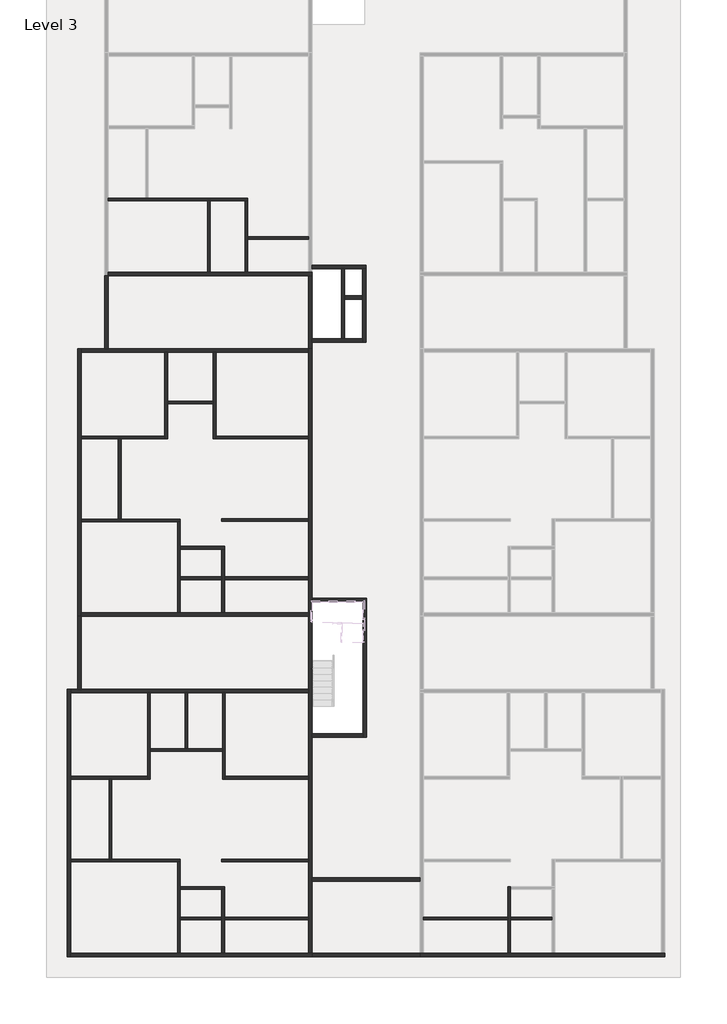
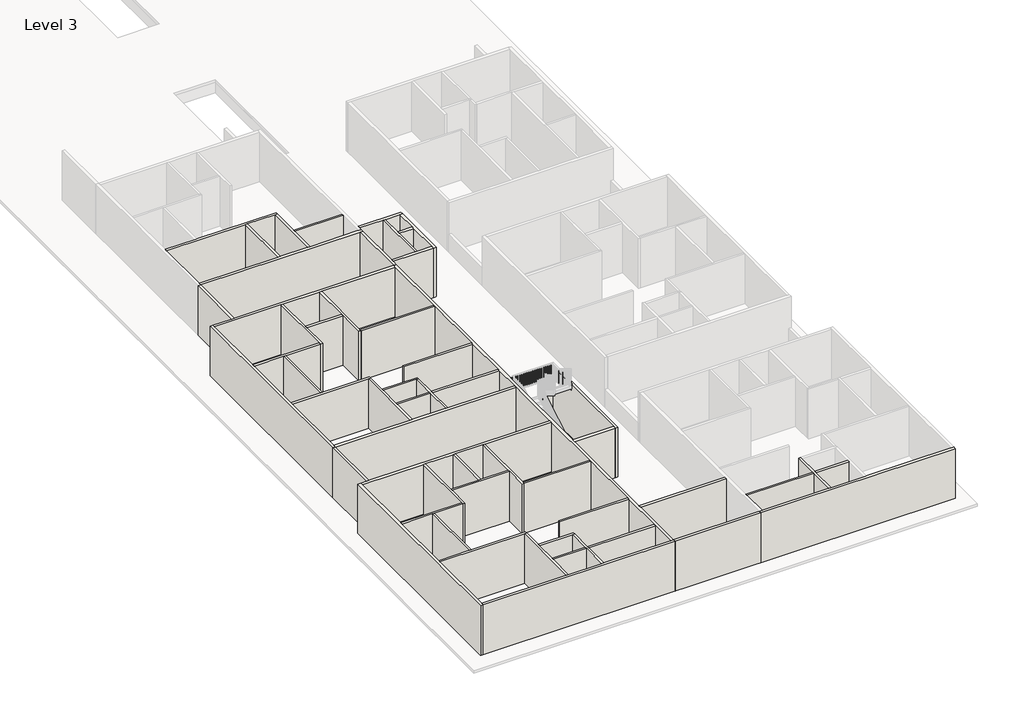
# One storey, part 1 of 8: 55 walls.
"""IFC4 building model written with IfcOpenShell, lengths in millimetres."""

from ifc_helpers import new_model, si_unit, frame, origin, place, context, project, spatial, polyline, outline, extrude, faceted_brep, element, save

model = new_model("IFC4")

# Units and contexts
model_context = context("Model", 3, world=origin())
ifc_project = project(units=[si_unit("LENGTHUNIT", "METRE", prefix="MILLI")], contexts=[model_context])

# Site, building, storey
site = spatial("IfcSite", under=ifc_project)
building = spatial("IfcBuilding", under=site)
storey = spatial("IfcBuildingStorey", under=building, Name="Level 3", Elevation=31330.6172466)

# Walls
placement = place(None, origin())
element("IfcWall", 1, ObjectType="4.5\"", at=placement, inside=storey, context=model_context, shape_type="Brep", body=[
    faceted_brep([(-12531.5544854, -1061.7344126, 31330.6172466), (-8188.1544854, -1061.7344126, 31330.6172466), (-8073.8544854, -1061.7344126, 31330.6172466), (-6549.8544854, -1061.7344126, 31330.6172466), (-6435.5544854, -1061.7344126, 31330.6172466), (-6435.5544854, -1061.7344126, 34378.6172466), (-6549.8544854, -1061.7344126, 34378.6172466), (-8073.8544854, -1061.7344126, 34378.6172466), (-8188.1544854, -1061.7344126, 34378.6172466), (-12531.5544854, -1061.7344126, 34378.6172466), (-12531.5544854, -947.4344126, 31330.6172466), (-12531.5544854, -947.4344126, 34378.6172466), (-10907.2415084, -947.4344126, 34378.6172466), (-10792.9415084, -947.4344126, 34378.6172466), (-6435.5544854, -947.4344126, 34378.6172466), (-6435.5544854, -947.4344126, 31330.6172466), (-10792.9415084, -947.4344126, 31330.6172466), (-10907.2415084, -947.4344126, 31330.6172466)], [[[0, 1, 2, 3, 4, 5, 6, 7, 8, 9]], [[10, 11, 12, 13, 14, 15, 16, 17]], [[4, 3, 2, 1, 0, 10, 17, 16, 15]], [[0, 9, 11, 10]], [[5, 4, 15, 14]], [[9, 8, 7, 6, 5, 14, 13, 12, 11]]]),
])
element("IfcWall", 2, ObjectType="4.5\"", at=placement, inside=storey, context=model_context, shape_type="Brep", body=[
    faceted_brep([(-6549.8544854, -1061.7344126, 31330.6172466), (-6549.8544854, -4185.9344126, 31330.6172466), (-6549.8544854, -4185.9344126, 34378.6172466), (-6549.8544854, -1061.7344126, 34378.6172466), (-6435.5544854, -1061.7344126, 31330.6172466), (-6435.5544854, -1061.7344126, 34378.6172466), (-6435.5544854, -2623.8344126, 34378.6172466), (-6435.5544854, -2738.1344126, 34378.6172466), (-6435.5544854, -4185.9344126, 34378.6172466), (-6435.5544854, -4185.9344126, 31330.6172466), (-6435.5544854, -2738.1344126, 31330.6172466), (-6435.5544854, -2623.8344126, 31330.6172466)], [[[0, 1, 2, 3]], [[4, 5, 6, 7, 8, 9, 10, 11]], [[1, 0, 4, 11, 10, 9]], [[0, 3, 5, 4]], [[2, 1, 9, 8]], [[3, 2, 8, 7, 6, 5]]]),
])
element("IfcWall", 3, ObjectType="4.5\"", at=placement, inside=storey, context=model_context, shape_type="SweptSolid", body=[
    extrude(outline(polyline([(-8188.1544854, -4185.9344126), (-8188.1544854, -1061.7344126), (-8073.8544854, -1061.7344126), (-8073.8544854, -4185.9344126), (-8188.1544854, -4185.9344126)])), frame((0.0, 0.0, 31330.6172466), z_axis=(0.0, 0.0, 1.0), x_axis=(1.0, 0.0, 0.0)), (0.0, 0.0, 1.0), 3048.0),
])
element("IfcWall", 4, ObjectType="4.5\"", at=placement, inside=storey, context=model_context, shape_type="SweptSolid", body=[
    extrude(outline(polyline([(-6435.5544854, -2623.8344126), (-3769.8415084, -2623.8344126), (-3769.8415084, -2738.1344126), (-6435.5544854, -2738.1344126), (-6435.5544854, -2623.8344126)])), frame((0.0, 0.0, 31330.6172466), z_axis=(0.0, 0.0, 1.0), x_axis=(1.0, 0.0, 0.0)), (0.0, 0.0, 1.0), 3048.0),
])
element("IfcWall", 5, ObjectType="4.5\"", at=placement, inside=storey, context=model_context, shape_type="Brep", body=[
    faceted_brep([(-10061.4044854, -7691.1344126, 31330.6172466), (-10061.4044854, -11348.7344126, 31330.6172466), (-10061.4044854, -11463.0344126, 31330.6172466), (-10061.4044854, -11463.0344126, 34378.6172466), (-10061.4044854, -11348.7344126, 34378.6172466), (-10061.4044854, -7691.1344126, 34378.6172466), (-9947.1044854, -7691.1344126, 31330.6172466), (-9947.1044854, -7691.1344126, 34378.6172466), (-9947.1044854, -9824.7344126, 34378.6172466), (-9947.1044854, -9939.0344126, 34378.6172466), (-9947.1044854, -11463.0344126, 34378.6172466), (-9947.1044854, -11463.0344126, 31330.6172466), (-9947.1044854, -9939.0344126, 31330.6172466), (-9947.1044854, -9824.7344126, 31330.6172466)], [[[0, 1, 2, 3, 4, 5]], [[6, 7, 8, 9, 10, 11, 12, 13]], [[2, 1, 0, 6, 13, 12, 11]], [[0, 5, 7, 6]], [[3, 2, 11, 10]], [[5, 4, 3, 10, 9, 8, 7]]]),
])
element("IfcWall", 6, ObjectType="4.5\"", at=placement, inside=storey, context=model_context, shape_type="Brep", body=[
    faceted_brep([(-10061.4044854, -11348.7344126, 31330.6172466), (-13719.0044854, -11348.7344126, 31330.6172466), (-13719.0044854, -11348.7344126, 34378.6172466), (-10061.4044854, -11348.7344126, 34378.6172466), (-10061.4044854, -11463.0344126, 31330.6172466), (-10061.4044854, -11463.0344126, 34378.6172466), (-11980.3915084, -11463.0344126, 34378.6172466), (-12094.6915084, -11463.0344126, 34378.6172466), (-13719.0044854, -11463.0344126, 34378.6172466), (-13719.0044854, -11463.0344126, 31330.6172466), (-12094.6915084, -11463.0344126, 31330.6172466), (-11980.3915084, -11463.0344126, 31330.6172466)], [[[0, 1, 2, 3]], [[4, 5, 6, 7, 8, 9, 10, 11]], [[1, 0, 4, 11, 10, 9]], [[0, 3, 5, 4]], [[2, 1, 9, 8]], [[3, 2, 8, 7, 6, 5]]]),
])
element("IfcWall", 7, ObjectType="4.5\"", at=placement, inside=storey, context=model_context, shape_type="SweptSolid", body=[
    extrude(outline(polyline([(-12094.6915084, -14968.2344126), (-12094.6915084, -11463.0344126), (-11980.3915084, -11463.0344126), (-11980.3915084, -14968.2344126), (-12094.6915084, -14968.2344126)])), frame((0.0, 0.0, 31330.6172466), z_axis=(0.0, 0.0, 1.0), x_axis=(1.0, 0.0, 0.0)), (0.0, 0.0, 1.0), 3048.0),
])
element("IfcWall", 8, ObjectType="4.5\"", at=placement, inside=storey, context=model_context, shape_type="Brep", body=[
    faceted_brep([(-13719.0044854, -15095.2344126, 31330.6172466), (-9510.2415084, -15095.2344126, 31330.6172466), (-9395.9415084, -15095.2344126, 31330.6172466), (-9395.9415084, -15095.2344126, 34378.6172466), (-9510.2415084, -15095.2344126, 34378.6172466), (-13719.0044854, -15095.2344126, 34378.6172466), (-13719.0044854, -14980.9344126, 31330.6172466), (-13719.0044854, -14980.9344126, 34378.6172466), (-9395.9415084, -14980.9344126, 34378.6172466), (-9395.9415084, -14980.9344126, 31330.6172466)], [[[0, 1, 2, 3, 4, 5]], [[6, 7, 8, 9]], [[2, 1, 0, 6, 9]], [[0, 5, 7, 6]], [[3, 2, 9, 8]], [[5, 4, 3, 8, 7]]]),
])
element("IfcWall", 9, ObjectType="4.5\"", at=placement, inside=storey, context=model_context, shape_type="Brep", body=[
    faceted_brep([(-9510.2415084, -15095.2344126, 31330.6172466), (-9510.2415084, -19070.3344126, 31330.6172466), (-9510.2415084, -19070.3344126, 34378.6172466), (-9510.2415084, -15095.2344126, 34378.6172466), (-9395.9415084, -15095.2344126, 31330.6172466), (-9395.9415084, -15095.2344126, 34378.6172466), (-9395.9415084, -16174.7344126, 34378.6172466), (-9395.9415084, -16289.0344126, 34378.6172466), (-9395.9415084, -17508.2344126, 34378.6172466), (-9395.9415084, -17622.5344126, 34378.6172466), (-9395.9415084, -19070.3344126, 34378.6172466), (-9395.9415084, -19070.3344126, 31330.6172466), (-9395.9415084, -17622.5344126, 31330.6172466), (-9395.9415084, -17508.2344126, 31330.6172466), (-9395.9415084, -16289.0344126, 31330.6172466), (-9395.9415084, -16174.7344126, 31330.6172466)], [[[0, 1, 2, 3]], [[4, 5, 6, 7, 8, 9, 10, 11, 12, 13, 14, 15]], [[1, 0, 4, 15, 14, 13, 12, 11]], [[0, 3, 5, 4]], [[2, 1, 11, 10]], [[3, 2, 10, 9, 8, 7, 6, 5]]]),
])
element("IfcWall", 10, ObjectType="4.5\"", at=placement, inside=storey, context=model_context, shape_type="Brep", body=[
    faceted_brep([(-9395.9415084, -16289.0344126, 31330.6172466), (-7567.1415084, -16289.0344126, 31330.6172466), (-7452.8415084, -16289.0344126, 31330.6172466), (-7452.8415084, -16289.0344126, 34378.6172466), (-7567.1415084, -16289.0344126, 34378.6172466), (-9395.9415084, -16289.0344126, 34378.6172466), (-9395.9415084, -16174.7344126, 31330.6172466), (-9395.9415084, -16174.7344126, 34378.6172466), (-7452.8415084, -16174.7344126, 34378.6172466), (-7452.8415084, -16174.7344126, 31330.6172466)], [[[0, 1, 2, 3, 4, 5]], [[6, 7, 8, 9]], [[2, 1, 0, 6, 9]], [[0, 5, 7, 6]], [[3, 2, 9, 8]], [[5, 4, 3, 8, 7]]]),
])
element("IfcWall", 11, ObjectType="4.5\"", at=placement, inside=storey, context=model_context, shape_type="Brep", body=[
    faceted_brep([(-7567.1415084, -16289.0344126, 31330.6172466), (-7567.1415084, -17508.2344126, 31330.6172466), (-7567.1415084, -17622.5344126, 31330.6172466), (-7567.1415084, -19070.3344126, 31330.6172466), (-7567.1415084, -19070.3344126, 34378.6172466), (-7567.1415084, -17622.5344126, 34378.6172466), (-7567.1415084, -17508.2344126, 34378.6172466), (-7567.1415084, -16289.0344126, 34378.6172466), (-7452.8415084, -16289.0344126, 31330.6172466), (-7452.8415084, -16289.0344126, 34378.6172466), (-7452.8415084, -17508.2344126, 34378.6172466), (-7452.8415084, -17622.5344126, 34378.6172466), (-7452.8415084, -19070.3344126, 34378.6172466), (-7452.8415084, -19070.3344126, 31330.6172466), (-7452.8415084, -17622.5344126, 31330.6172466), (-7452.8415084, -17508.2344126, 31330.6172466)], [[[0, 1, 2, 3, 4, 5, 6, 7]], [[8, 9, 10, 11, 12, 13, 14, 15]], [[3, 2, 1, 0, 8, 15, 14, 13]], [[0, 7, 9, 8]], [[4, 3, 13, 12]], [[7, 6, 5, 4, 12, 11, 10, 9]]]),
])
element("IfcWall", 12, ObjectType="4.5\"", at=placement, inside=storey, context=model_context, shape_type="SweptSolid", body=[
    extrude(outline(polyline([(-7567.1415084, -17622.5344126), (-9395.9415084, -17622.5344126), (-9395.9415084, -17508.2344126), (-7567.1415084, -17508.2344126), (-7567.1415084, -17622.5344126)])), frame((0.0, 0.0, 31330.6172466), z_axis=(0.0, 0.0, 1.0), x_axis=(1.0, 0.0, 0.0)), (0.0, 0.0, 1.0), 3048.0),
])
element("IfcWall", 13, ObjectType="4.5\"", at=placement, inside=storey, context=model_context, shape_type="SweptSolid", body=[
    extrude(outline(polyline([(-3769.8415084, -17622.5344126), (-7452.8415084, -17622.5344126), (-7452.8415084, -17508.2344126), (-3769.8415084, -17508.2344126), (-3769.8415084, -17622.5344126)])), frame((0.0, 0.0, 31330.6172466), z_axis=(0.0, 0.0, 1.0), x_axis=(1.0, 0.0, 0.0)), (0.0, 0.0, 1.0), 3048.0),
])
element("IfcWall", 14, ObjectType="4.5\"", at=placement, inside=storey, context=model_context, shape_type="SweptSolid", body=[
    extrude(outline(polyline([(-7567.1415084, -14968.2344126), (-3769.8415084, -14968.2344126), (-3769.8415084, -15082.5344126), (-7567.1415084, -15082.5344126), (-7567.1415084, -14968.2344126)])), frame((0.0, 0.0, 31330.6172466), z_axis=(0.0, 0.0, 1.0), x_axis=(1.0, 0.0, 0.0)), (0.0, 0.0, 1.0), 3048.0),
])
element("IfcWall", 15, ObjectType="4.5\"", at=placement, inside=storey, context=model_context, shape_type="SweptSolid", body=[
    extrude(outline(polyline([(-7940.5044854, -9939.0344126), (-9947.1044854, -9939.0344126), (-9947.1044854, -9824.7344126), (-7940.5044854, -9824.7344126), (-7940.5044854, -9939.0344126)])), frame((0.0, 0.0, 31330.6172466), z_axis=(0.0, 0.0, 1.0), x_axis=(1.0, 0.0, 0.0)), (0.0, 0.0, 1.0), 3048.0),
])
element("IfcWall", 16, ObjectType="4.5\"", at=placement, inside=storey, context=model_context, shape_type="Brep", body=[
    faceted_brep([(-7940.5044854, -7691.1344126, 31330.6172466), (-7940.5044854, -9824.7344126, 31330.6172466), (-7940.5044854, -9939.0344126, 31330.6172466), (-7940.5044854, -11463.0344126, 31330.6172466), (-7940.5044854, -11463.0344126, 34378.6172466), (-7940.5044854, -9939.0344126, 34378.6172466), (-7940.5044854, -9824.7344126, 34378.6172466), (-7940.5044854, -7691.1344126, 34378.6172466), (-7826.2044854, -7691.1344126, 31330.6172466), (-7826.2044854, -7691.1344126, 34378.6172466), (-7826.2044854, -11348.7344126, 34378.6172466), (-7826.2044854, -11463.0344126, 34378.6172466), (-7826.2044854, -11463.0344126, 31330.6172466), (-7826.2044854, -11348.7344126, 31330.6172466)], [[[0, 1, 2, 3, 4, 5, 6, 7]], [[8, 9, 10, 11, 12, 13]], [[3, 2, 1, 0, 8, 13, 12]], [[0, 7, 9, 8]], [[4, 3, 12, 11]], [[7, 6, 5, 4, 11, 10, 9]]]),
])
element("IfcWall", 17, ObjectType="4.5\"", at=placement, inside=storey, context=model_context, shape_type="SweptSolid", body=[
    extrude(outline(polyline([(-3769.8415084, -11463.0344126), (-7826.2044854, -11463.0344126), (-7826.2044854, -11348.7344126), (-3769.8415084, -11348.7344126), (-3769.8415084, -11463.0344126)])), frame((0.0, 0.0, 31330.6172466), z_axis=(0.0, 0.0, 1.0), x_axis=(1.0, 0.0, 0.0)), (0.0, 0.0, 1.0), 3048.0),
])
element("IfcWall", 18, ObjectType="4.5\"", at=placement, inside=storey, context=model_context, shape_type="Brep", body=[
    faceted_brep([(-10818.3415084, -22575.5344126, 31330.6172466), (-10818.3415084, -26233.1344126, 31330.6172466), (-10818.3415084, -26347.4344126, 31330.6172466), (-10818.3415084, -26347.4344126, 34378.6172466), (-10818.3415084, -26233.1344126, 34378.6172466), (-10818.3415084, -22575.5344126, 34378.6172466), (-10704.0415084, -22575.5344126, 31330.6172466), (-10704.0415084, -22575.5344126, 34378.6172466), (-10704.0415084, -25013.9344126, 34378.6172466), (-10704.0415084, -25128.2344126, 34378.6172466), (-10704.0415084, -26347.4344126, 34378.6172466), (-10704.0415084, -26347.4344126, 31330.6172466), (-10704.0415084, -25128.2344126, 31330.6172466), (-10704.0415084, -25013.9344126, 31330.6172466)], [[[0, 1, 2, 3, 4, 5]], [[6, 7, 8, 9, 10, 11, 12, 13]], [[2, 1, 0, 6, 13, 12, 11]], [[0, 5, 7, 6]], [[3, 2, 11, 10]], [[5, 4, 3, 10, 9, 8, 7]]]),
])
element("IfcWall", 19, ObjectType="4.5\"", at=placement, inside=storey, context=model_context, shape_type="Brep", body=[
    faceted_brep([(-10818.3415084, -26233.1344126, 31330.6172466), (-14171.1415084, -26233.1344126, 31330.6172466), (-14171.1415084, -26233.1344126, 34378.6172466), (-10818.3415084, -26233.1344126, 34378.6172466), (-10818.3415084, -26347.4344126, 31330.6172466), (-10818.3415084, -26347.4344126, 34378.6172466), (-12380.4415084, -26347.4344126, 34378.6172466), (-12494.7415084, -26347.4344126, 34378.6172466), (-14171.1415084, -26347.4344126, 34378.6172466), (-14171.1415084, -26347.4344126, 31330.6172466), (-12494.7415084, -26347.4344126, 31330.6172466), (-12380.4415084, -26347.4344126, 31330.6172466)], [[[0, 1, 2, 3]], [[4, 5, 6, 7, 8, 9, 10, 11]], [[1, 0, 4, 11, 10, 9]], [[0, 3, 5, 4]], [[2, 1, 9, 8]], [[3, 2, 8, 7, 6, 5]]]),
])
element("IfcWall", 20, ObjectType="4.5\"", at=placement, inside=storey, context=model_context, shape_type="SweptSolid", body=[
    extrude(outline(polyline([(-9180.0415084, -25013.9344126), (-9180.0415084, -22575.5344126), (-9065.7415084, -22575.5344126), (-9065.7415084, -25013.9344126), (-9180.0415084, -25013.9344126)])), frame((0.0, 0.0, 31330.6172466), z_axis=(0.0, 0.0, 1.0), x_axis=(1.0, 0.0, 0.0)), (0.0, 0.0, 1.0), 3048.0),
])
element("IfcWall", 21, ObjectType="4.5\"", at=placement, inside=storey, context=model_context, shape_type="Brep", body=[
    faceted_brep([(-10704.0415084, -25128.2344126, 31330.6172466), (-7541.7415084, -25128.2344126, 31330.6172466), (-7541.7415084, -25128.2344126, 34378.6172466), (-10704.0415084, -25128.2344126, 34378.6172466), (-10704.0415084, -25013.9344126, 31330.6172466), (-10704.0415084, -25013.9344126, 34378.6172466), (-9180.0415084, -25013.9344126, 34378.6172466), (-9065.7415084, -25013.9344126, 34378.6172466), (-7541.7415084, -25013.9344126, 34378.6172466), (-7541.7415084, -25013.9344126, 31330.6172466), (-9065.7415084, -25013.9344126, 31330.6172466), (-9180.0415084, -25013.9344126, 31330.6172466)], [[[0, 1, 2, 3]], [[4, 5, 6, 7, 8, 9, 10, 11]], [[1, 0, 4, 11, 10, 9]], [[0, 3, 5, 4]], [[2, 1, 9, 8]], [[3, 2, 8, 7, 6, 5]]]),
])
element("IfcWall", 22, ObjectType="4.5\"", at=placement, inside=storey, context=model_context, shape_type="Brep", body=[
    faceted_brep([(-7541.7415084, -22575.5344126, 31330.6172466), (-7541.7415084, -25013.9344126, 31330.6172466), (-7541.7415084, -25128.2344126, 31330.6172466), (-7541.7415084, -26347.4344126, 31330.6172466), (-7541.7415084, -26347.4344126, 34378.6172466), (-7541.7415084, -25128.2344126, 34378.6172466), (-7541.7415084, -25013.9344126, 34378.6172466), (-7541.7415084, -22575.5344126, 34378.6172466), (-7427.4415084, -22575.5344126, 31330.6172466), (-7427.4415084, -22575.5344126, 34378.6172466), (-7427.4415084, -26233.1344126, 34378.6172466), (-7427.4415084, -26347.4344126, 34378.6172466), (-7427.4415084, -26347.4344126, 31330.6172466), (-7427.4415084, -26233.1344126, 31330.6172466)], [[[0, 1, 2, 3, 4, 5, 6, 7]], [[8, 9, 10, 11, 12, 13]], [[3, 2, 1, 0, 8, 13, 12]], [[0, 7, 9, 8]], [[4, 3, 12, 11]], [[7, 6, 5, 4, 11, 10, 9]]]),
])
element("IfcWall", 23, ObjectType="4.5\"", at=placement, inside=storey, context=model_context, shape_type="SweptSolid", body=[
    extrude(outline(polyline([(-3769.8415084, -26347.4344126), (-7427.4415084, -26347.4344126), (-7427.4415084, -26233.1344126), (-3769.8415084, -26233.1344126), (-3769.8415084, -26347.4344126)])), frame((0.0, 0.0, 31330.6172466), z_axis=(0.0, 0.0, 1.0), x_axis=(1.0, 0.0, 0.0)), (0.0, 0.0, 1.0), 3048.0),
])
element("IfcWall", 24, ObjectType="4.5\"", at=placement, inside=storey, context=model_context, shape_type="SweptSolid", body=[
    extrude(outline(polyline([(-12494.7415084, -29852.6344126), (-12494.7415084, -26347.4344126), (-12380.4415084, -26347.4344126), (-12380.4415084, -29852.6344126), (-12494.7415084, -29852.6344126)])), frame((0.0, 0.0, 31330.6172466), z_axis=(0.0, 0.0, 1.0), x_axis=(1.0, 0.0, 0.0)), (0.0, 0.0, 1.0), 3048.0),
])
element("IfcWall", 25, ObjectType="4.5\"", at=placement, inside=storey, context=model_context, shape_type="Brep", body=[
    faceted_brep([(-14171.1415084, -29966.9344126, 31330.6172466), (-9510.2415084, -29966.9344126, 31330.6172466), (-9395.9415084, -29966.9344126, 31330.6172466), (-9395.9415084, -29966.9344126, 34378.6172466), (-9510.2415084, -29966.9344126, 34378.6172466), (-14171.1415084, -29966.9344126, 34378.6172466), (-14171.1415084, -29852.6344126, 31330.6172466), (-14171.1415084, -29852.6344126, 34378.6172466), (-12494.7415084, -29852.6344126, 34378.6172466), (-12380.4415084, -29852.6344126, 34378.6172466), (-9395.9415084, -29852.6344126, 34378.6172466), (-9395.9415084, -29852.6344126, 31330.6172466), (-12380.4415084, -29852.6344126, 31330.6172466), (-12494.7415084, -29852.6344126, 31330.6172466)], [[[0, 1, 2, 3, 4, 5]], [[6, 7, 8, 9, 10, 11, 12, 13]], [[2, 1, 0, 6, 13, 12, 11]], [[0, 5, 7, 6]], [[3, 2, 11, 10]], [[5, 4, 3, 10, 9, 8, 7]]]),
])
element("IfcWall", 26, ObjectType="4.5\"", at=placement, inside=storey, context=model_context, shape_type="Brep", body=[
    faceted_brep([(-9510.2415084, -29966.9344126, 31330.6172466), (-9510.2415084, -33954.7344126, 31330.6172466), (-9510.2415084, -33954.7344126, 34378.6172466), (-9510.2415084, -29966.9344126, 34378.6172466), (-9395.9415084, -29966.9344126, 31330.6172466), (-9395.9415084, -29966.9344126, 34378.6172466), (-9395.9415084, -31059.1344126, 34378.6172466), (-9395.9415084, -31173.4344126, 34378.6172466), (-9395.9415084, -32392.6344126, 34378.6172466), (-9395.9415084, -32506.9344126, 34378.6172466), (-9395.9415084, -33954.7344126, 34378.6172466), (-9395.9415084, -33954.7344126, 31330.6172466), (-9395.9415084, -32506.9344126, 31330.6172466), (-9395.9415084, -32392.6344126, 31330.6172466), (-9395.9415084, -31173.4344126, 31330.6172466), (-9395.9415084, -31059.1344126, 31330.6172466)], [[[0, 1, 2, 3]], [[4, 5, 6, 7, 8, 9, 10, 11, 12, 13, 14, 15]], [[1, 0, 4, 15, 14, 13, 12, 11]], [[0, 3, 5, 4]], [[2, 1, 11, 10]], [[3, 2, 10, 9, 8, 7, 6, 5]]]),
])
element("IfcWall", 27, ObjectType="4.5\"", at=placement, inside=storey, context=model_context, shape_type="Brep", body=[
    faceted_brep([(-9395.9415084, -31173.4344126, 31330.6172466), (-7567.1415084, -31173.4344126, 31330.6172466), (-7452.8415084, -31173.4344126, 31330.6172466), (-7452.8415084, -31173.4344126, 34378.6172466), (-7567.1415084, -31173.4344126, 34378.6172466), (-9395.9415084, -31173.4344126, 34378.6172466), (-9395.9415084, -31059.1344126, 31330.6172466), (-9395.9415084, -31059.1344126, 34378.6172466), (-7452.8415084, -31059.1344126, 34378.6172466), (-7452.8415084, -31059.1344126, 31330.6172466)], [[[0, 1, 2, 3, 4, 5]], [[6, 7, 8, 9]], [[2, 1, 0, 6, 9]], [[0, 5, 7, 6]], [[3, 2, 9, 8]], [[5, 4, 3, 8, 7]]]),
])
element("IfcWall", 28, ObjectType="4.5\"", at=placement, inside=storey, context=model_context, shape_type="Brep", body=[
    faceted_brep([(-7567.1415084, -31173.4344126, 31330.6172466), (-7567.1415084, -32392.6344126, 31330.6172466), (-7567.1415084, -32506.9344126, 31330.6172466), (-7567.1415084, -33954.7344126, 31330.6172466), (-7567.1415084, -33954.7344126, 34378.6172466), (-7567.1415084, -32506.9344126, 34378.6172466), (-7567.1415084, -32392.6344126, 34378.6172466), (-7567.1415084, -31173.4344126, 34378.6172466), (-7452.8415084, -31173.4344126, 31330.6172466), (-7452.8415084, -31173.4344126, 34378.6172466), (-7452.8415084, -32392.6344126, 34378.6172466), (-7452.8415084, -32506.9344126, 34378.6172466), (-7452.8415084, -33954.7344126, 34378.6172466), (-7452.8415084, -33954.7344126, 31330.6172466), (-7452.8415084, -32506.9344126, 31330.6172466), (-7452.8415084, -32392.6344126, 31330.6172466)], [[[0, 1, 2, 3, 4, 5, 6, 7]], [[8, 9, 10, 11, 12, 13, 14, 15]], [[3, 2, 1, 0, 8, 15, 14, 13]], [[0, 7, 9, 8]], [[4, 3, 13, 12]], [[7, 6, 5, 4, 12, 11, 10, 9]]]),
])
element("IfcWall", 29, ObjectType="4.5\"", at=placement, inside=storey, context=model_context, shape_type="SweptSolid", body=[
    extrude(outline(polyline([(-3769.8415084, -32392.6344126), (-3769.8415084, -32506.9344126), (-7452.8415084, -32506.9344126), (-7452.8415084, -32392.6344126), (-3769.8415084, -32392.6344126)])), frame((0.0, 0.0, 31330.6172466), z_axis=(0.0, 0.0, 1.0), x_axis=(1.0, 0.0, 0.0)), (0.0, 0.0, 1.0), 3048.0),
    extrude(outline(polyline([(-9395.9415084, -32506.9344126), (-9395.9415084, -32392.6344126), (-7567.1415084, -32392.6344126), (-7567.1415084, -32506.9344126), (-9395.9415084, -32506.9344126)])), frame((0.0, 0.0, 31330.6172466), z_axis=(0.0, 0.0, 1.0), x_axis=(1.0, 0.0, 0.0)), (0.0, 0.0, 1.0), 3048.0),
])
element("IfcWall", 30, ObjectType="4.5\"", at=placement, inside=storey, context=model_context, shape_type="SweptSolid", body=[
    extrude(outline(polyline([(-7567.1415084, -29852.6344126), (-3769.8415084, -29852.6344126), (-3769.8415084, -29966.9344126), (-7567.1415084, -29966.9344126), (-7567.1415084, -29852.6344126)])), frame((0.0, 0.0, 31330.6172466), z_axis=(0.0, 0.0, 1.0), x_axis=(1.0, 0.0, 0.0)), (0.0, 0.0, 1.0), 3048.0),
])
element("IfcWall", 31, ObjectType="4.5\"", at=placement, inside=storey, context=model_context, shape_type="SweptSolid", body=[
    extrude(outline(polyline([(4942.3584916, -32506.9344126), (1259.3584916, -32506.9344126), (1259.3584916, -32392.6344126), (4942.3584916, -32392.6344126), (4942.3584916, -32506.9344126)])), frame((0.0, 0.0, 31330.6172466), z_axis=(0.0, 0.0, 1.0), x_axis=(1.0, 0.0, 0.0)), (0.0, 0.0, 1.0), 3048.0),
])
element("IfcWall", 32, ObjectType="4.5\"", at=placement, inside=storey, context=model_context, shape_type="Brep", body=[
    faceted_brep([(4942.3584916, -31059.1344126, 31330.6172466), (4942.3584916, -32392.6344126, 31330.6172466), (4942.3584916, -32506.9344126, 31330.6172466), (4942.3584916, -33954.7344126, 31330.6172466), (4942.3584916, -33954.7344126, 34378.6172466), (4942.3584916, -32506.9344126, 34378.6172466), (4942.3584916, -32392.6344126, 34378.6172466), (4942.3584916, -31059.1344126, 34378.6172466), (5056.6584916, -31059.1344126, 31330.6172466), (5056.6584916, -31059.1344126, 34378.6172466), (5056.6584916, -31173.4344126, 34378.6172466), (5056.6584916, -32392.6344126, 34378.6172466), (5056.6584916, -32506.9344126, 34378.6172466), (5056.6584916, -33954.7344126, 34378.6172466), (5056.6584916, -33954.7344126, 31330.6172466), (5056.6584916, -32506.9344126, 31330.6172466), (5056.6584916, -32392.6344126, 31330.6172466), (5056.6584916, -31173.4344126, 31330.6172466)], [[[0, 1, 2, 3, 4, 5, 6, 7]], [[8, 9, 10, 11, 12, 13, 14, 15, 16, 17]], [[3, 2, 1, 0, 8, 17, 16, 15, 14]], [[4, 3, 14, 13]], [[0, 7, 9, 8]], [[7, 6, 5, 4, 13, 12, 11, 10, 9]]]),
])
element("IfcWall", 33, ObjectType="4.5\"", at=placement, inside=storey, context=model_context, shape_type="SweptSolid", body=[
    extrude(outline(polyline([(6885.4584916, -32506.9344126), (5056.6584916, -32506.9344126), (5056.6584916, -32392.6344126), (6885.4584916, -32392.6344126), (6885.4584916, -32506.9344126)])), frame((0.0, 0.0, 31330.6172466), z_axis=(0.0, 0.0, 1.0), x_axis=(1.0, 0.0, 0.0)), (0.0, 0.0, 1.0), 3048.0),
])
element("IfcWall", 34, ObjectType="4.5\"", at=placement, inside=storey, context=model_context, shape_type="Brep", body=[
    faceted_brep([(-2207.6738684, -7082.6751812, 31330.6172466), (-2207.6738684, -5366.3479894, 31330.6172466), (-2207.6738684, -5213.9479894, 31330.6172466), (-2207.6738684, -4034.6751812, 31330.6172466), (-2207.6738684, -4034.6751812, 34378.6172466), (-2207.6738684, -5213.9479894, 34378.6172466), (-2207.6738684, -5366.3479894, 34378.6172466), (-2207.6738684, -7082.6751812, 34378.6172466), (-2321.9738684, -7082.6751812, 31330.6172466), (-2321.9738684, -7082.6751812, 34378.6172466), (-2321.9738684, -4034.6751812, 34378.6172466), (-2321.9738684, -4034.6751812, 31330.6172466)], [[[0, 1, 2, 3, 4, 5, 6, 7]], [[8, 9, 10, 11]], [[3, 2, 1, 0, 8, 11]], [[7, 6, 5, 4, 10, 9]], [[4, 3, 11, 10]], [[0, 7, 9, 8]]]),
])
element("IfcWall", 35, ObjectType="6\"", at=placement, inside=storey, context=model_context, shape_type="Brep", body=[
    faceted_brep([(-12531.5544854, -4338.3344126, 31330.6172466), (-3769.8415084, -4338.3344126, 31330.6172466), (-3617.4415084, -4338.3344126, 31330.6172466), (-3617.4415084, -4338.3344126, 34378.6172466), (-3769.8415084, -4338.3344126, 34378.6172466), (-12531.5544854, -4338.3344126, 34378.6172466), (-12531.5544854, -4185.9344126, 31330.6172466), (-12531.5544854, -4185.9344126, 34378.6172466), (-8188.1544854, -4185.9344126, 34378.6172466), (-8073.8544854, -4185.9344126, 34378.6172466), (-6549.8544854, -4185.9344126, 34378.6172466), (-6435.5544854, -4185.9344126, 34378.6172466), (-3769.8415084, -4185.9344126, 34378.6172466), (-3617.4415084, -4185.9344126, 34378.6172466), (-3617.4415084, -4185.9344126, 31330.6172466), (-3769.8415084, -4185.9344126, 31330.6172466), (-6435.5544854, -4185.9344126, 31330.6172466), (-6549.8544854, -4185.9344126, 31330.6172466), (-8073.8544854, -4185.9344126, 31330.6172466), (-8188.1544854, -4185.9344126, 31330.6172466)], [[[0, 1, 2, 3, 4, 5]], [[6, 7, 8, 9, 10, 11, 12, 13, 14, 15, 16, 17, 18, 19]], [[2, 1, 0, 6, 19, 18, 17, 16, 15, 14]], [[0, 5, 7, 6]], [[3, 2, 14, 13]], [[5, 4, 3, 13, 12, 11, 10, 9, 8, 7]]]),
])
element("IfcWall", 36, ObjectType="6\"", at=placement, inside=storey, context=model_context, shape_type="Brep", body=[
    faceted_brep([(-13871.4044854, -7538.7344126, 31330.6172466), (-13871.4044854, -19222.7344126, 31330.6172466), (-13871.4044854, -19222.7344126, 34378.6172466), (-13871.4044854, -7538.7344126, 34378.6172466), (-13719.0044854, -7538.7344126, 31330.6172466), (-13719.0044854, -7538.7344126, 34378.6172466), (-13719.0044854, -7691.1344126, 34378.6172466), (-13719.0044854, -11348.7344126, 34378.6172466), (-13719.0044854, -11463.0344126, 34378.6172466), (-13719.0044854, -14980.9344126, 34378.6172466), (-13719.0044854, -15095.2344126, 34378.6172466), (-13719.0044854, -19070.3344126, 34378.6172466), (-13719.0044854, -19222.7344126, 34378.6172466), (-13719.0044854, -19222.7344126, 31330.6172466), (-13719.0044854, -19070.3344126, 31330.6172466), (-13719.0044854, -15095.2344126, 31330.6172466), (-13719.0044854, -14980.9344126, 31330.6172466), (-13719.0044854, -11463.0344126, 31330.6172466), (-13719.0044854, -11348.7344126, 31330.6172466), (-13719.0044854, -7691.1344126, 31330.6172466)], [[[0, 1, 2, 3]], [[4, 5, 6, 7, 8, 9, 10, 11, 12, 13, 14, 15, 16, 17, 18, 19]], [[1, 0, 4, 19, 18, 17, 16, 15, 14, 13]], [[2, 1, 13, 12]], [[0, 3, 5, 4]], [[3, 2, 12, 11, 10, 9, 8, 7, 6, 5]]]),
])
element("IfcWall", 37, ObjectType="6\"", at=placement, inside=storey, context=model_context, shape_type="Brep", body=[
    faceted_brep([(-13719.0044854, -19222.7344126, 31330.6172466), (-3769.8415084, -19222.7344126, 31330.6172466), (-3769.8415084, -19222.7344126, 34378.6172466), (-13719.0044854, -19222.7344126, 34378.6172466), (-13719.0044854, -19070.3344126, 31330.6172466), (-13719.0044854, -19070.3344126, 34378.6172466), (-9510.2415084, -19070.3344126, 34378.6172466), (-9395.9415084, -19070.3344126, 34378.6172466), (-7567.1415084, -19070.3344126, 34378.6172466), (-7452.8415084, -19070.3344126, 34378.6172466), (-3769.8415084, -19070.3344126, 34378.6172466), (-3769.8415084, -19070.3344126, 31330.6172466), (-7452.8415084, -19070.3344126, 31330.6172466), (-7567.1415084, -19070.3344126, 31330.6172466), (-9395.9415084, -19070.3344126, 31330.6172466), (-9510.2415084, -19070.3344126, 31330.6172466)], [[[0, 1, 2, 3]], [[4, 5, 6, 7, 8, 9, 10, 11, 12, 13, 14, 15]], [[1, 0, 4, 15, 14, 13, 12, 11]], [[0, 3, 5, 4]], [[2, 1, 11, 10]], [[3, 2, 10, 9, 8, 7, 6, 5]]]),
])
element("IfcWall", 38, ObjectType="6\"", at=placement, inside=storey, context=model_context, shape_type="Brep", body=[
    faceted_brep([(-3617.4415084, -33954.7344126, 31330.6172466), (-3617.4415084, -30820.9325185, 31330.6172466), (-3617.4415084, -30668.5325185, 31330.6172466), (-3617.4415084, -24525.9851539, 31330.6172466), (-3617.4415084, -24373.5851539, 31330.6172466), (-3617.4415084, -18582.3851539, 31330.6172466), (-3617.4415084, -18429.9851539, 31330.6172466), (-3617.4415084, -7538.7344126, 31330.6172466), (-3617.4415084, -7538.7344126, 34378.6172466), (-3617.4415084, -18429.9851539, 34378.6172466), (-3617.4415084, -18582.3851539, 34378.6172466), (-3617.4415084, -24373.5851539, 34378.6172466), (-3617.4415084, -24525.9851539, 34378.6172466), (-3617.4415084, -30668.5325185, 34378.6172466), (-3617.4415084, -30820.9325185, 34378.6172466), (-3617.4415084, -33954.7344126, 34378.6172466), (-3769.8415084, -33954.7344126, 31330.6172466), (-3769.8415084, -33954.7344126, 34378.6172466), (-3769.8415084, -32506.9344126, 34378.6172466), (-3769.8415084, -32392.6344126, 34378.6172466), (-3769.8415084, -29966.9344126, 34378.6172466), (-3769.8415084, -29852.6344126, 34378.6172466), (-3769.8415084, -26347.4344126, 34378.6172466), (-3769.8415084, -26233.1344126, 34378.6172466), (-3769.8415084, -22575.5344126, 34378.6172466), (-3769.8415084, -22423.1344126, 34378.6172466), (-3769.8415084, -19222.7344126, 34378.6172466), (-3769.8415084, -19070.3344126, 34378.6172466), (-3769.8415084, -17622.5344126, 34378.6172466), (-3769.8415084, -17508.2344126, 34378.6172466), (-3769.8415084, -15082.5344126, 34378.6172466), (-3769.8415084, -14968.2344126, 34378.6172466), (-3769.8415084, -11463.0344126, 34378.6172466), (-3769.8415084, -11348.7344126, 34378.6172466), (-3769.8415084, -7691.1344126, 34378.6172466), (-3769.8415084, -7538.7344126, 34378.6172466), (-3769.8415084, -7538.7344126, 31330.6172466), (-3769.8415084, -7691.1344126, 31330.6172466), (-3769.8415084, -11348.7344126, 31330.6172466), (-3769.8415084, -11463.0344126, 31330.6172466), (-3769.8415084, -14968.2344126, 31330.6172466), (-3769.8415084, -15082.5344126, 31330.6172466), (-3769.8415084, -17508.2344126, 31330.6172466), (-3769.8415084, -17622.5344126, 31330.6172466), (-3769.8415084, -19070.3344126, 31330.6172466), (-3769.8415084, -19222.7344126, 31330.6172466), (-3769.8415084, -22423.1344126, 31330.6172466), (-3769.8415084, -22575.5344126, 31330.6172466), (-3769.8415084, -26233.1344126, 31330.6172466), (-3769.8415084, -26347.4344126, 31330.6172466), (-3769.8415084, -29852.6344126, 31330.6172466), (-3769.8415084, -29966.9344126, 31330.6172466), (-3769.8415084, -32392.6344126, 31330.6172466), (-3769.8415084, -32506.9344126, 31330.6172466)], [[[0, 1, 2, 3, 4, 5, 6, 7, 8, 9, 10, 11, 12, 13, 14, 15]], [[16, 17, 18, 19, 20, 21, 22, 23, 24, 25, 26, 27, 28, 29, 30, 31, 32, 33, 34, 35, 36, 37, 38, 39, 40, 41, 42, 43, 44, 45, 46, 47, 48, 49, 50, 51, 52, 53]], [[7, 6, 5, 4, 3, 2, 1, 0, 16, 53, 52, 51, 50, 49, 48, 47, 46, 45, 44, 43, 42, 41, 40, 39, 38, 37, 36]], [[8, 7, 36, 35]], [[0, 15, 17, 16]], [[15, 14, 13, 12, 11, 10, 9, 8, 35, 34, 33, 32, 31, 30, 29, 28, 27, 26, 25, 24, 23, 22, 21, 20, 19, 18, 17]]]),
])
element("IfcWall", 39, ObjectType="6\"", at=placement, inside=storey, context=model_context, shape_type="Brep", body=[
    faceted_brep([(-3769.8415084, -7538.7344126, 31330.6172466), (-12531.5544854, -7538.7344126, 31330.6172466), (-12683.9544854, -7538.7344126, 31330.6172466), (-13719.0044854, -7538.7344126, 31330.6172466), (-13719.0044854, -7538.7344126, 34378.6172466), (-12683.9544854, -7538.7344126, 34378.6172466), (-12531.5544854, -7538.7344126, 34378.6172466), (-3769.8415084, -7538.7344126, 34378.6172466), (-3769.8415084, -7691.1344126, 31330.6172466), (-3769.8415084, -7691.1344126, 34378.6172466), (-7826.2044854, -7691.1344126, 34378.6172466), (-7940.5044854, -7691.1344126, 34378.6172466), (-9947.1044854, -7691.1344126, 34378.6172466), (-10061.4044854, -7691.1344126, 34378.6172466), (-13719.0044854, -7691.1344126, 34378.6172466), (-13719.0044854, -7691.1344126, 31330.6172466), (-10061.4044854, -7691.1344126, 31330.6172466), (-9947.1044854, -7691.1344126, 31330.6172466), (-7940.5044854, -7691.1344126, 31330.6172466), (-7826.2044854, -7691.1344126, 31330.6172466)], [[[0, 1, 2, 3, 4, 5, 6, 7]], [[8, 9, 10, 11, 12, 13, 14, 15, 16, 17, 18, 19]], [[3, 2, 1, 0, 8, 19, 18, 17, 16, 15]], [[0, 7, 9, 8]], [[4, 3, 15, 14]], [[7, 6, 5, 4, 14, 13, 12, 11, 10, 9]]]),
])
element("IfcWall", 40, ObjectType="6\"", at=placement, inside=storey, context=model_context, shape_type="Brep", body=[
    faceted_brep([(-14323.5415084, -22423.1344126, 31330.6172466), (-14323.5415084, -34107.1344126, 31330.6172466), (-14323.5415084, -34107.1344126, 34378.6172466), (-14323.5415084, -22423.1344126, 34378.6172466), (-14171.1415084, -22423.1344126, 31330.6172466), (-14171.1415084, -22423.1344126, 34378.6172466), (-14171.1415084, -22575.5344126, 34378.6172466), (-14171.1415084, -26233.1344126, 34378.6172466), (-14171.1415084, -26347.4344126, 34378.6172466), (-14171.1415084, -29852.6344126, 34378.6172466), (-14171.1415084, -29966.9344126, 34378.6172466), (-14171.1415084, -33954.7344126, 34378.6172466), (-14171.1415084, -34107.1344126, 34378.6172466), (-14171.1415084, -34107.1344126, 31330.6172466), (-14171.1415084, -33954.7344126, 31330.6172466), (-14171.1415084, -29966.9344126, 31330.6172466), (-14171.1415084, -29852.6344126, 31330.6172466), (-14171.1415084, -26347.4344126, 31330.6172466), (-14171.1415084, -26233.1344126, 31330.6172466), (-14171.1415084, -22575.5344126, 31330.6172466)], [[[0, 1, 2, 3]], [[4, 5, 6, 7, 8, 9, 10, 11, 12, 13, 14, 15, 16, 17, 18, 19]], [[1, 0, 4, 19, 18, 17, 16, 15, 14, 13]], [[2, 1, 13, 12]], [[0, 3, 5, 4]], [[3, 2, 12, 11, 10, 9, 8, 7, 6, 5]]]),
])
element("IfcWall", 41, ObjectType="6\"", at=placement, inside=storey, context=model_context, shape_type="Brep", body=[
    faceted_brep([(-14171.1415084, -34107.1344126, 31330.6172466), (-3617.4415084, -34107.1344126, 31330.6172466), (-3617.4415084, -34107.1344126, 34378.6172466), (-14171.1415084, -34107.1344126, 34378.6172466), (-14171.1415084, -33954.7344126, 31330.6172466), (-14171.1415084, -33954.7344126, 34378.6172466), (-9510.2415084, -33954.7344126, 34378.6172466), (-9395.9415084, -33954.7344126, 34378.6172466), (-7567.1415084, -33954.7344126, 34378.6172466), (-7452.8415084, -33954.7344126, 34378.6172466), (-3769.8415084, -33954.7344126, 34378.6172466), (-3617.4415084, -33954.7344126, 34378.6172466), (-3617.4415084, -33954.7344126, 31330.6172466), (-3769.8415084, -33954.7344126, 31330.6172466), (-7452.8415084, -33954.7344126, 31330.6172466), (-7567.1415084, -33954.7344126, 31330.6172466), (-9395.9415084, -33954.7344126, 31330.6172466), (-9510.2415084, -33954.7344126, 31330.6172466)], [[[0, 1, 2, 3]], [[4, 5, 6, 7, 8, 9, 10, 11, 12, 13, 14, 15, 16, 17]], [[1, 0, 4, 17, 16, 15, 14, 13, 12]], [[0, 3, 5, 4]], [[2, 1, 12, 11]], [[3, 2, 11, 10, 9, 8, 7, 6, 5]]]),
])
element("IfcWall", 42, ObjectType="6\"", at=placement, inside=storey, context=model_context, shape_type="Brep", body=[
    faceted_brep([(-3769.8415084, -22423.1344126, 31330.6172466), (-13719.0044854, -22423.1344126, 31330.6172466), (-13871.4044854, -22423.1344126, 31330.6172466), (-14171.1415084, -22423.1344126, 31330.6172466), (-14171.1415084, -22423.1344126, 34378.6172466), (-13871.4044854, -22423.1344126, 34378.6172466), (-13719.0044854, -22423.1344126, 34378.6172466), (-3769.8415084, -22423.1344126, 34378.6172466), (-3769.8415084, -22575.5344126, 31330.6172466), (-3769.8415084, -22575.5344126, 34378.6172466), (-7427.4415084, -22575.5344126, 34378.6172466), (-7541.7415084, -22575.5344126, 34378.6172466), (-9065.7415084, -22575.5344126, 34378.6172466), (-9180.0415084, -22575.5344126, 34378.6172466), (-10704.0415084, -22575.5344126, 34378.6172466), (-10818.3415084, -22575.5344126, 34378.6172466), (-14171.1415084, -22575.5344126, 34378.6172466), (-14171.1415084, -22575.5344126, 31330.6172466), (-10818.3415084, -22575.5344126, 31330.6172466), (-10704.0415084, -22575.5344126, 31330.6172466), (-9180.0415084, -22575.5344126, 31330.6172466), (-9065.7415084, -22575.5344126, 31330.6172466), (-7541.7415084, -22575.5344126, 31330.6172466), (-7427.4415084, -22575.5344126, 31330.6172466)], [[[0, 1, 2, 3, 4, 5, 6, 7]], [[8, 9, 10, 11, 12, 13, 14, 15, 16, 17, 18, 19, 20, 21, 22, 23]], [[3, 2, 1, 0, 8, 23, 22, 21, 20, 19, 18, 17]], [[0, 7, 9, 8]], [[4, 3, 17, 16]], [[7, 6, 5, 4, 16, 15, 14, 13, 12, 11, 10, 9]]]),
])
element("IfcWall", 43, ObjectType="6\"", at=placement, inside=storey, context=model_context, shape_type="Brep", body=[
    faceted_brep([(1106.9584916, -34107.1344126, 31330.6172466), (11813.0584916, -34107.1344126, 31330.6172466), (11813.0584916, -34107.1344126, 34378.6172466), (1106.9584916, -34107.1344126, 34378.6172466), (1106.9584916, -33954.7344126, 31330.6172466), (1106.9584916, -33954.7344126, 34378.6172466), (1259.3584916, -33954.7344126, 34378.6172466), (4942.3584916, -33954.7344126, 34378.6172466), (5056.6584916, -33954.7344126, 34378.6172466), (6885.4584916, -33954.7344126, 34378.6172466), (6999.7584916, -33954.7344126, 34378.6172466), (11660.6584916, -33954.7344126, 34378.6172466), (11813.0584916, -33954.7344126, 34378.6172466), (11813.0584916, -33954.7344126, 31330.6172466), (11660.6584916, -33954.7344126, 31330.6172466), (6999.7584916, -33954.7344126, 31330.6172466), (6885.4584916, -33954.7344126, 31330.6172466), (5056.6584916, -33954.7344126, 31330.6172466), (4942.3584916, -33954.7344126, 31330.6172466), (1259.3584916, -33954.7344126, 31330.6172466)], [[[0, 1, 2, 3]], [[4, 5, 6, 7, 8, 9, 10, 11, 12, 13, 14, 15, 16, 17, 18, 19]], [[1, 0, 4, 19, 18, 17, 16, 15, 14, 13]], [[2, 1, 13, 12]], [[0, 3, 5, 4]], [[3, 2, 12, 11, 10, 9, 8, 7, 6, 5]]]),
])
element("IfcWall", 44, ObjectType="6\"", at=placement, inside=storey, context=model_context, shape_type="Brep", body=[
    faceted_brep([(-3617.4415084, -18582.3851539, 31330.6172466), (-1382.2415084, -18582.3851539, 31330.6172466), (-1229.8415084, -18582.3851539, 31330.6172466), (-1229.8415084, -18582.3851539, 34378.6172466), (-1382.2415084, -18582.3851539, 34378.6172466), (-3617.4415084, -18582.3851539, 34378.6172466), (-3617.4415084, -18429.9851539, 31330.6172466), (-3617.4415084, -18429.9851539, 34378.6172466), (-1229.8415084, -18429.9851539, 34378.6172466), (-1229.8415084, -18429.9851539, 31330.6172466)], [[[0, 1, 2, 3, 4, 5]], [[6, 7, 8, 9]], [[2, 1, 0, 6, 9]], [[5, 4, 3, 8, 7]], [[0, 5, 7, 6]], [[3, 2, 9, 8]]]),
])
element("IfcWall", 45, ObjectType="6\"", at=placement, inside=storey, context=model_context, shape_type="Brep", body=[
    faceted_brep([(-1382.2415084, -18582.3851539, 31330.6172466), (-1382.2415084, -24373.5851539, 31330.6172466), (-1382.2415084, -24525.9851539, 31330.6172466), (-1382.2415084, -24525.9851539, 34378.6172466), (-1382.2415084, -24373.5851539, 34378.6172466), (-1382.2415084, -18582.3851539, 34378.6172466), (-1229.8415084, -18582.3851539, 31330.6172466), (-1229.8415084, -18582.3851539, 34378.6172466), (-1229.8415084, -24525.9851539, 34378.6172466), (-1229.8415084, -24525.9851539, 31330.6172466)], [[[0, 1, 2, 3, 4, 5]], [[6, 7, 8, 9]], [[2, 1, 0, 6, 9]], [[5, 4, 3, 8, 7]], [[0, 5, 7, 6]], [[3, 2, 9, 8]]]),
])
element("IfcWall", 46, ObjectType="6\"", at=placement, inside=storey, context=model_context, shape_type="SweptSolid", body=[
    extrude(outline(polyline([(-3617.4415084, -24373.5851539), (-1382.2415084, -24373.5851539), (-1382.2415084, -24525.9851539), (-3617.4415084, -24525.9851539), (-3617.4415084, -24373.5851539)])), frame((0.0, 0.0, 31330.6172466), z_axis=(0.0, 0.0, 1.0), x_axis=(1.0, 0.0, 0.0)), (0.0, 0.0, 1.0), 3048.0),
])
element("IfcWall", 47, ObjectType="6\"", at=placement, inside=storey, context=model_context, shape_type="Brep", body=[
    faceted_brep([(-3769.8415084, -4338.3344126, 31330.6172466), (-3769.8415084, -7538.7344126, 31330.6172466), (-3769.8415084, -7538.7344126, 34378.6172466), (-3769.8415084, -4338.3344126, 34378.6172466), (-3617.4415084, -4338.3344126, 31330.6172466), (-3617.4415084, -4338.3344126, 34378.6172466), (-3617.4415084, -7082.6751812, 34378.6172466), (-3617.4415084, -7235.0751812, 34378.6172466), (-3617.4415084, -7538.7344126, 34378.6172466), (-3617.4415084, -7538.7344126, 31330.6172466), (-3617.4415084, -7235.0751812, 31330.6172466), (-3617.4415084, -7082.6751812, 31330.6172466)], [[[0, 1, 2, 3]], [[4, 5, 6, 7, 8, 9, 10, 11]], [[1, 0, 4, 11, 10, 9]], [[0, 3, 5, 4]], [[2, 1, 9, 8]], [[3, 2, 8, 7, 6, 5]]]),
])
element("IfcWall", 48, ObjectType="6\"", at=placement, inside=storey, context=model_context, shape_type="Brep", body=[
    faceted_brep([(-3617.4415084, -4034.6751812, 31330.6172466), (-2321.9738684, -4034.6751812, 31330.6172466), (-2207.6738684, -4034.6751812, 31330.6172466), (-1407.6415084, -4034.6751812, 31330.6172466), (-1255.2415084, -4034.6751812, 31330.6172466), (-1255.2415084, -4034.6751812, 34378.6172466), (-1407.6415084, -4034.6751812, 34378.6172466), (-2207.6738684, -4034.6751812, 34378.6172466), (-2321.9738684, -4034.6751812, 34378.6172466), (-3617.4415084, -4034.6751812, 34378.6172466), (-3617.4415084, -3882.2751812, 31330.6172466), (-3617.4415084, -3882.2751812, 34378.6172466), (-1255.2415084, -3882.2751812, 34378.6172466), (-1255.2415084, -3882.2751812, 31330.6172466)], [[[0, 1, 2, 3, 4, 5, 6, 7, 8, 9]], [[10, 11, 12, 13]], [[4, 3, 2, 1, 0, 10, 13]], [[9, 8, 7, 6, 5, 12, 11]], [[0, 9, 11, 10]], [[5, 4, 13, 12]]]),
])
element("IfcWall", 49, ObjectType="6\"", at=placement, inside=storey, context=model_context, shape_type="Brep", body=[
    faceted_brep([(-1407.6415084, -4034.6751812, 31330.6172466), (-1407.6415084, -5213.9479894, 31330.6172466), (-1407.6415084, -5366.3479894, 31330.6172466), (-1407.6415084, -7082.6751812, 31330.6172466), (-1407.6415084, -7235.0751812, 31330.6172466), (-1407.6415084, -7235.0751812, 34378.6172466), (-1407.6415084, -7082.6751812, 34378.6172466), (-1407.6415084, -5366.3479894, 34378.6172466), (-1407.6415084, -5213.9479894, 34378.6172466), (-1407.6415084, -4034.6751812, 34378.6172466), (-1255.2415084, -4034.6751812, 31330.6172466), (-1255.2415084, -4034.6751812, 34378.6172466), (-1255.2415084, -7235.0751812, 34378.6172466), (-1255.2415084, -7235.0751812, 31330.6172466)], [[[0, 1, 2, 3, 4, 5, 6, 7, 8, 9]], [[10, 11, 12, 13]], [[4, 3, 2, 1, 0, 10, 13]], [[9, 8, 7, 6, 5, 12, 11]], [[0, 9, 11, 10]], [[5, 4, 13, 12]]]),
])
element("IfcWall", 50, ObjectType="6\"", at=placement, inside=storey, context=model_context, shape_type="Brep", body=[
    faceted_brep([(-1407.6415084, -7082.6751812, 31330.6172466), (-2207.6738684, -7082.6751812, 31330.6172466), (-2321.9738684, -7082.6751812, 31330.6172466), (-3617.4415084, -7082.6751812, 31330.6172466), (-3617.4415084, -7082.6751812, 34378.6172466), (-2321.9738684, -7082.6751812, 34378.6172466), (-2207.6738684, -7082.6751812, 34378.6172466), (-1407.6415084, -7082.6751812, 34378.6172466), (-1407.6415084, -7235.0751812, 31330.6172466), (-1407.6415084, -7235.0751812, 34378.6172466), (-3617.4415084, -7235.0751812, 34378.6172466), (-3617.4415084, -7235.0751812, 31330.6172466)], [[[0, 1, 2, 3, 4, 5, 6, 7]], [[8, 9, 10, 11]], [[3, 2, 1, 0, 8, 11]], [[7, 6, 5, 4, 10, 9]], [[0, 7, 9, 8]], [[4, 3, 11, 10]]]),
])
element("IfcWall", 51, ObjectType="6\"", at=placement, inside=storey, context=model_context, shape_type="SweptSolid", body=[
    extrude(outline(polyline([(-2207.6738684, -5213.9479894), (-1407.6415084, -5213.9479894), (-1407.6415084, -5366.3479894), (-2207.6738684, -5366.3479894), (-2207.6738684, -5213.9479894)])), frame((0.0, 0.0, 31330.6172466), z_axis=(0.0, 0.0, 1.0), x_axis=(1.0, 0.0, 0.0)), (0.0, 0.0, 1.0), 3048.0),
])
element("IfcWall", 52, ObjectType="6\" 2", at=placement, inside=storey, context=model_context, shape_type="SweptSolid", body=[
    extrude(outline(polyline([(1106.9584916, -34107.1344126), (-3617.4415084, -34107.1344126), (-3617.4415084, -33954.7344126), (1106.9584916, -33954.7344126), (1106.9584916, -34107.1344126)])), frame((0.0, 0.0, 31330.6172466), z_axis=(0.0, 0.0, 1.0), x_axis=(1.0, 0.0, 0.0)), (0.0, 0.0, 1.0), 3048.0),
])
element("IfcWall", 53, ObjectType="6\" 2", at=placement, inside=storey, context=model_context, shape_type="SweptSolid", body=[
    extrude(outline(polyline([(-3617.4415084, -30668.5325185), (1106.9584916, -30668.5325185), (1106.9584916, -30820.9325185), (-3617.4415084, -30820.9325185), (-3617.4415084, -30668.5325185)])), frame((0.0, 0.0, 31330.6172466), z_axis=(0.0, 0.0, 1.0), x_axis=(1.0, 0.0, 0.0)), (0.0, 0.0, 1.0), 3048.0),
])
element("IfcWall", 54, ObjectType="6\" 2", at=placement, inside=storey, context=model_context, shape_type="SweptSolid", body=[
    extrude(outline(polyline([(-13871.4044854, -22423.1344126), (-13871.4044854, -19222.7344126), (-13719.0044854, -19222.7344126), (-13719.0044854, -22423.1344126), (-13871.4044854, -22423.1344126)])), frame((0.0, 0.0, 31330.6172466), z_axis=(0.0, 0.0, 1.0), x_axis=(1.0, 0.0, 0.0)), (0.0, 0.0, 1.0), 3048.0),
])
element("IfcWall", 55, ObjectType="6\" 2", at=placement, inside=storey, context=model_context, shape_type="SweptSolid", body=[
    extrude(outline(polyline([(-12683.9544854, -7538.7344126), (-12683.9544854, -4338.3344126), (-12531.5544854, -4338.3344126), (-12531.5544854, -7538.7344126), (-12683.9544854, -7538.7344126)])), frame((0.0, 0.0, 31330.6172466), z_axis=(0.0, 0.0, 1.0), x_axis=(1.0, 0.0, 0.0)), (0.0, 0.0, 1.0), 3048.0),
])

save(model, "model.ifc")

# Revit data of these elements
# Type "4.5\""
#   Assembly Code = "B2010"
#   Layers, outside or top first: 0' - 4 1/2" "WALLS" (function 1)
# Type "6\""
#   Assembly Code = "B2010"
#   Layers, outside or top first: 0' - 6" "WALLS" (function 1)
# Type "6\" 2"
#   Assembly Code = "B2010"
#   Layers, outside or top first: 0' - 6" "4'" (function 1)
# Elements 1, 2, 3, 4, 5, 6, 7, 8, 9, 10, 11, 12, 13, 14, 15, 16, 17, 18, 19, 20, 21, 22, 23, 24, 25, 26, 27, 28, 29, 30, 31, 32, 33, 34 (IfcWall, "4.5\"")
#   Top Offset = 0' - 0"
#   Base Offset = 0' - 0"
#   Unconnected Height = 10' - 0"
#   wall height = 10' - 0"
#   Phase Created = New Construction
#   Base Constraint = Level 3
#   Materials on its faces: "WALLS"
# Elements 35, 36, 37, 38, 39, 40, 41, 42, 43, 44, 45, 46, 47, 48, 49, 50, 51 (IfcWall, "6\"")
#   Top Offset = 0' - 0"
#   Base Offset = 0' - 0"
#   Unconnected Height = 10' - 0"
#   wall height = 10' - 0"
#   Phase Created = New Construction
#   Base Constraint = Level 3
#   Materials on its faces: "WALLS"
# Elements 52, 53, 54, 55 (IfcWall, "6\" 2")
#   Top Offset = 0' - 0"
#   Base Offset = 0' - 0"
#   Unconnected Height = 10' - 0"
#   wall height = 10' - 0"
#   Phase Created = New Construction
#   Base Constraint = Level 3
#   Materials on its faces: "4'"
# Materials
#   "WALLS": class "Generic", colour RGB 120 120 120, transparency 0, Cost = 0
#   "4'": class "Generic", colour RGB 120 120 120, transparency 0, Cost = 0
